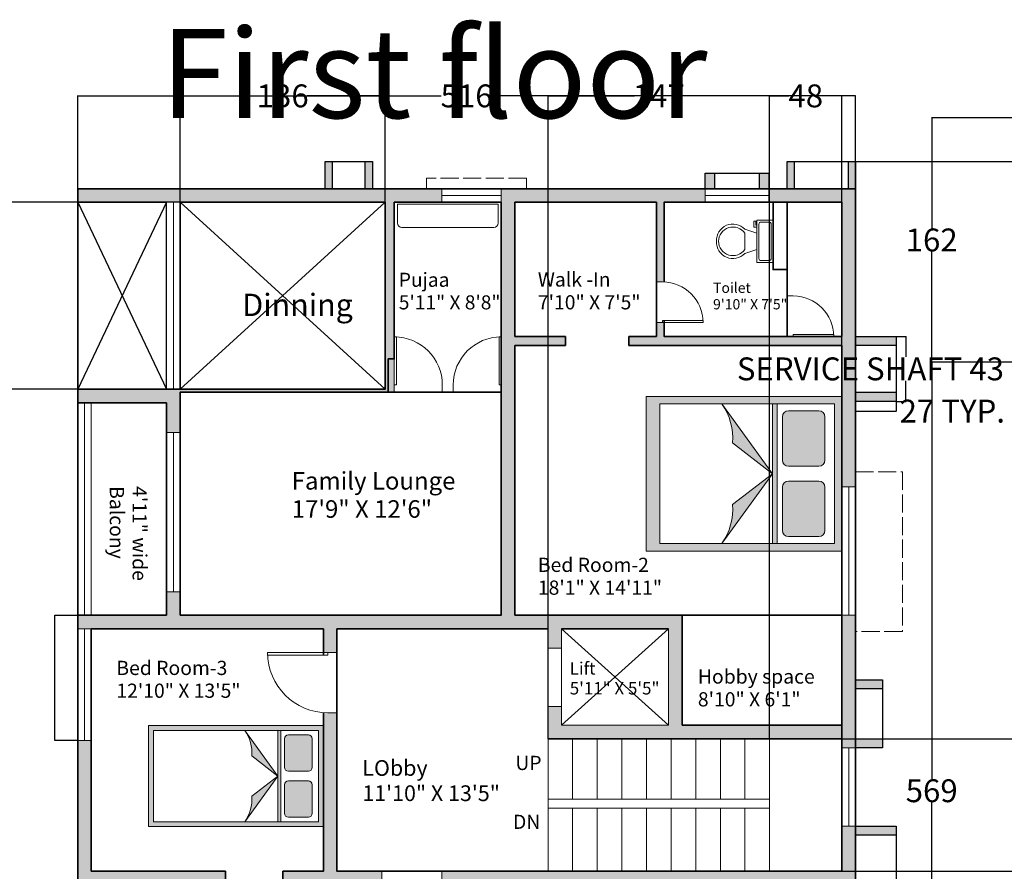
# Model space of a CAD drawing. Units: inches. Extents: x -828 to 1568, y -491 to 539.
# Tile 5 of 6: x 241 to 895, y -110 to 455. Entities that reach past the tile are written whole.
import ezdxf

# ---------------------------------------------------------------- set-up
doc = ezdxf.new("R2010")
doc.units = ezdxf.units.IN
doc.header["$MEASUREMENT"] = 0
doc.linetypes.add('ACAD_ISO02W100', pattern=[15, 12, -3])
for name, color, linetype, lineweight in [('A-ANNO-DIMS', 2, 'Continuous', 18), ('A-ANNO-TEXT', 7, 'Continuous', 18), ('A-ANNO-TITL', 7, 'Continuous', 35), ('A-AREA-IDEN', 7, 'Continuous', 18), ('A-DOOR', 3, 'Continuous', 18), ('A-FLOR-CASE', 9, 'Continuous', 18), ('A-FLOR-EDGE', 7, 'Continuous', 25), ('A-FLOR-EVTR', 4, 'Continuous', 18), ('A-FLOR-FIXT', 9, 'Continuous', 18), ('A-FLOR-OPEN', 8, 'Continuous', 13), ('A-FLOR-OVHD', 116, 'ACAD_ISO02W100', 13), ('A-FLOR-SHFT', 7, 'Continuous', 25), ('A-FLOR-STRS', 7, 'Continuous', 18), ('A-FURN', 8, 'Continuous', 18), ('A-FURN-PATT', 253, 'Continuous', 13), ('A-GLAZ', 4, 'Continuous', 18), ('A-WALL', 7, 'Continuous', 35), ('A-WALL-PATT', 8, 'Continuous', 13)]:
    doc.layers.add(name, color=color, linetype=linetype, lineweight=lineweight)
doc.styles.get("Standard").update_dxf_attribs({"font": 'arial.ttf'})
doc.dimstyles.get("Standard").update_dxf_attribs({"dimtxt": 15.18, "dimasz": 0.18, "dimexe": 0.18, "dimexo": 0.0625, "dimgap": 0.09, "dimtad": 0, "dimtih": 1, "dimtoh": 1, "dimdec": 0, "dimzin": 0, "dimdsep": 46, "dimlunit": 3, "dimtxsty": 'Standard', "dimcen": 0.09, "dimadec": 0, "dimazin": 0, "dimtfac": 1, "dimtdec": 0, "dimtofl": 0, "dimtmove": 0, "dimatfit": 3, "dimfxl": 1, "dimtolj": 1, "dimtzin": 0, "dimarcsym": 0})

# ---------------------------------------------------------------- blocks, each defined once
blk = doc.blocks.new('*U2')
for p, q in [((0, 0), (0, -6)), ((40, 0), (40, -6))]:
    blk.add_line(p, q)
blk.add_lwpolyline([(0, 0), (0, 40), (1.75, 40), (1.75, 0)], close=True)
blk.add_arc((0, 0), 40, 0, 90)
blk = doc.blocks.new('*U6')
for p, q in [((9.5, -6), (9.5, -2)), ((-10, -8.5), (-8, -8.5)), ((-10, -9.5), (-10, -8.5)), ((-7, -9.5), (-10, -9.5)), ((-8, -8.5), (-8, -8)), ((-7, -8), (-7, -9.5)), ((-4, -8), (-6, -14)), ((4, -8), (6, -14)), ((4, -14), (-4, -14))]:
    blk.add_line(p, q)
blk.add_lwpolyline([(10.5, -8), (10.5, 0), (-10.5, 0), (-10.5, -8)], close=True)
for points in [[(-9.5, -2), (-9.5, -6)], [(8.5, -1), (-8.5, -1)], [(-8.5, -7), (8.5, -7)]]:
    blk.add_lwpolyline(points)
for centre, radius, start, end in [((-8.625, -1.875), 0.8839, 81.8699, 188.1301), ((8.625, -1.875), 0.8839, 351.8699, 98.1301), ((-8.625, -6.125), 0.8839, 171.869898, 278.1301), ((8.625, -6.125), 0.8839, 261.8699, 8.1301), ((-0.4772, -19.9188), 8.0953, 133.01722, 273.38), ((0.0374, -19.8731), 7.127, 124.50543, 269.7), ((-0.0373, -19.8731), 7.127, 270.3, 55.4946), ((0.4773, -19.9188), 8.0953, 266.62, 46.9828)]:
    blk.add_arc(centre, radius, start, end)
blk = doc.blocks.new('SERVICE-SHAFT-43')
blk.add_line((26.86, 37.12), (26.86, 6))
for points in [[(0, 43.12), (26.86, 43.12), (26.86, 37.12), (0, 37.12)], [(0, 6), (26.86, 6), (26.86, 0), (0, 0)]]:
    blk.add_lwpolyline(points, close=True)
blk = doc.blocks.new('BED-FRAME-TURNBACK')
h = blk.add_hatch(color=256)
h.dxf.hatch_style = 1
h.paths.add_polyline_path([(0, 0), (115.93, 0), (115.93, 67.12), (0, 67.12)])
h.paths.add_polyline_path([(3.27, 63.85), (112.66, 63.85), (112.66, 3.27), (3.27, 3.27)], flags=16)
h = blk.add_hatch(color=256)
h.dxf.hatch_style = 1
h.paths.add_polyline_path([(63.77, 63.85, -0.182673), (68.41, 46.96), (85.81, 33.56)])
h.paths.add_polyline_path([(85.81, 33.56), (68.41, 20.16, -0.182673), (63.77, 3.27)])
h = blk.add_hatch(color=256)
h.dxf.hatch_style = 1
h.paths.add_polyline_path([(87.78, 33.56), (85.81, 33.56), (85.81, 3.27), (87.78, 3.27)])
h.paths.add_polyline_path([(87.78, 63.85), (85.81, 63.85), (85.81, 33.56), (87.78, 33.56)])
for p, q in [((85.81, 33.56), (63.77, 63.85)), ((85.81, 3.27), (85.81, 63.85)), ((87.78, 3.27), (87.78, 63.85)), ((85.81, 33.56), (68.41, 46.96))]:
    blk.add_line(p, q)
for points in [[(115.93, 0), (0, 0), (0, 67.12), (115.93, 67.12)], [(112.66, 3.27), (3.27, 3.27), (3.27, 63.85), (112.66, 63.85)]]:
    blk.add_lwpolyline(points, close=True)
blk.add_lwpolyline([(63.77, 3.27, 0.182673), (68.41, 20.16), (85.81, 33.56)], format="xyb", close=True)
blk.add_arc((43.75, 49.27), 24.77, 354.63295, 36.04187)
blk = doc.blocks.new('*D25')
at = {"layer": 'A-ANNO-DIMS', "color": 0, "lineweight": -2, "transparency": 16777216}
for p, q in [((822.84, 244.58), (829.43, 244.58)), ((829.25, 244.4), (829.25, 230.97)), ((829.25, 201.64), (829.25, 215.08)), ((822.84, 201.46), (829.43, 201.46))]:
    blk.add_line(p, q, dxfattribs=at)
at = {"layer": 'A-ANNO-DIMS', "color": 0, "lineweight": 20, "transparency": 16777216}
for points in [[(829.22, 244.4), (829.28, 244.4), (829.25, 244.58)], [(829.22, 201.64), (829.28, 201.64), (829.25, 201.46)]]:
    blk.add_solid(points, dxfattribs=at)
at = {"layer": 'DEFPOINTS', "color": 0, "lineweight": 20, "transparency": 16777216}
for p in [(822.78, 244.58), (829.25, 244.58), (822.78, 201.46)]:
    blk.add_point(p, dxfattribs=at)
at = {"layer": 'A-ANNO-DIMS', "color": 0, "transparency": 16777216, "insert": (829.25, 223.02), "char_height": 15.18, "attachment_point": 5}
blk.add_mtext('\\A1;SERVICE SHAFT 43 TYP.', dxfattribs=at)
blk = doc.blocks.new('*D26')
at = {"layer": 'A-ANNO-DIMS', "color": 0, "lineweight": -2, "transparency": 16777216}
for p, q in [((795.92, 201.4), (795.92, 194.82)), ((822.78, 201.4), (822.78, 194.82)), ((796.1, 195), (822.6, 195)), ((822.78, 195), (822.96, 195))]:
    blk.add_line(p, q, dxfattribs=at)
at = {"layer": 'A-ANNO-DIMS', "color": 0, "lineweight": 20, "transparency": 16777216}
for points in [[(796.1, 195.03), (796.1, 194.97), (795.92, 195)], [(822.6, 195.03), (822.6, 194.97), (822.78, 195)]]:
    blk.add_solid(points, dxfattribs=at)
at = {"layer": 'DEFPOINTS', "color": 0, "lineweight": 20, "transparency": 16777216}
for p in [(795.92, 201.46), (822.78, 201.46), (822.78, 195)]:
    blk.add_point(p, dxfattribs=at)
at = {"layer": 'A-ANNO-DIMS', "color": 0, "transparency": 16777216, "insert": (860.13, 195), "char_height": 15.18, "attachment_point": 5}
blk.add_mtext('\\A1;27 TYP.', dxfattribs=at)
blk = doc.blocks.new('*D40')
at = {"layer": 'A-ANNO-DIMS', "color": 0, "lineweight": -2, "transparency": 16777216}
for p, q in [((795.99, 360.63), (969.15, 360.63)), ((968.97, 360.45), (968.97, -20.38)), ((968.97, -416.57), (968.97, -35.74)), ((568.26, -416.75), (969.15, -416.75))]:
    blk.add_line(p, q, dxfattribs=at)
at = {"layer": 'A-ANNO-DIMS', "color": 0, "lineweight": 20, "transparency": 16777216}
for points in [[(968.94, 360.45), (969, 360.45), (968.97, 360.63)], [(968.94, -416.57), (969, -416.57), (968.97, -416.75)]]:
    blk.add_solid(points, dxfattribs=at)
at = {"layer": 'DEFPOINTS', "color": 0, "lineweight": 20, "transparency": 16777216}
for p in [(795.92, 360.63), (968.97, 360.63), (568.2, -416.75)]:
    blk.add_point(p, dxfattribs=at)
at = {"layer": 'A-ANNO-DIMS', "color": 0, "transparency": 16777216, "insert": (968.97, -28.06), "char_height": 15.18, "attachment_point": 5}
blk.add_mtext('\\A1;777.4', dxfattribs=at)
blk = doc.blocks.new('*D41')
at = {"layer": 'A-ANNO-DIMS', "color": 0, "lineweight": -2, "transparency": 16777216}
for p, q in [((279.92, 342.65), (279.92, 404.36)), ((280.1, 404.18), (521.07, 404.18)), ((795.74, 404.18), (554.78, 404.18)), ((795.92, 342.65), (795.92, 404.36))]:
    blk.add_line(p, q, dxfattribs=at)
at = {"layer": 'A-ANNO-DIMS', "color": 0, "lineweight": 20, "transparency": 16777216}
for points in [[(280.1, 404.21), (280.1, 404.15), (279.92, 404.18)], [(795.74, 404.21), (795.74, 404.15), (795.92, 404.18)]]:
    blk.add_solid(points, dxfattribs=at)
at = {"layer": 'DEFPOINTS', "color": 0, "lineweight": 20, "transparency": 16777216}
for p in [(795.92, 404.18), (279.92, 342.58), (795.92, 342.58)]:
    blk.add_point(p, dxfattribs=at)
at = {"layer": 'A-ANNO-DIMS', "color": 0, "transparency": 16777216, "insert": (537.92, 404.18), "char_height": 15.18, "attachment_point": 5}
blk.add_mtext('\\A1;516', dxfattribs=at)
blk = doc.blocks.new('*D42')
at = {"layer": 'A-ANNO-DIMS', "color": 0, "lineweight": -2, "transparency": 16777216}
for p, q in [((347.86, 209.58), (141.48, 209.58)), ((141.66, 209.4), (141.66, -76.07)), ((141.66, -377.24), (141.66, -91.76)), ((279.86, -377.42), (141.48, -377.42))]:
    blk.add_line(p, q, dxfattribs=at)
at = {"layer": 'A-ANNO-DIMS', "color": 0, "lineweight": 20, "transparency": 16777216}
for points in [[(141.63, 209.4), (141.69, 209.4), (141.66, 209.58)], [(141.63, -377.24), (141.69, -377.24), (141.66, -377.42)]]:
    blk.add_solid(points, dxfattribs=at)
at = {"layer": 'DEFPOINTS', "color": 0, "lineweight": 20, "transparency": 16777216}
for p in [(141.66, 209.58), (347.92, 209.58), (279.92, -377.42)]:
    blk.add_point(p, dxfattribs=at)
at = {"layer": 'A-ANNO-DIMS', "color": 0, "transparency": 16777216, "insert": (141.66, -83.92), "char_height": 15.18, "attachment_point": 5}
blk.add_mtext('\\A1;587', dxfattribs=at)
blk = doc.blocks.new('*D43')
at = {"layer": 'A-ANNO-DIMS', "color": 0, "lineweight": -2, "transparency": 16777216}
for p, q in [((347.92, 333.65), (347.92, 404.36)), ((348.1, 404.18), (399.78, 404.18)), ((483.74, 404.18), (432.06, 404.18)), ((483.92, 333.65), (483.92, 404.36))]:
    blk.add_line(p, q, dxfattribs=at)
at = {"layer": 'A-ANNO-DIMS', "color": 0, "lineweight": 20, "transparency": 16777216}
for points in [[(348.1, 404.21), (348.1, 404.15), (347.92, 404.18)], [(483.74, 404.21), (483.74, 404.15), (483.92, 404.18)]]:
    blk.add_solid(points, dxfattribs=at)
at = {"layer": 'DEFPOINTS', "color": 0, "lineweight": 20, "transparency": 16777216}
for p in [(483.92, 404.18), (347.92, 333.58), (483.92, 333.58)]:
    blk.add_point(p, dxfattribs=at)
at = {"layer": 'A-ANNO-DIMS', "color": 0, "transparency": 16777216, "insert": (415.92, 404.18), "char_height": 15.18, "attachment_point": 5}
blk.add_mtext('\\A1;136', dxfattribs=at)
blk = doc.blocks.new('*D44')
at = {"layer": 'A-ANNO-DIMS', "color": 0, "lineweight": -2, "transparency": 16777216}
for p, q in [((347.86, 333.58), (141.48, 333.58)), ((141.66, 333.4), (141.66, 279.3)), ((141.66, 209.76), (141.66, 263.87)), ((347.86, 209.58), (141.48, 209.58))]:
    blk.add_line(p, q, dxfattribs=at)
at = {"layer": 'A-ANNO-DIMS', "color": 0, "lineweight": 20, "transparency": 16777216}
for points in [[(141.63, 333.4), (141.69, 333.4), (141.66, 333.58)], [(141.63, 209.76), (141.69, 209.76), (141.66, 209.58)]]:
    blk.add_solid(points, dxfattribs=at)
at = {"layer": 'DEFPOINTS', "color": 0, "lineweight": 20, "transparency": 16777216}
for p in [(141.66, 333.58), (347.92, 333.58), (347.92, 209.58)]:
    blk.add_point(p, dxfattribs=at)
at = {"layer": 'A-ANNO-DIMS', "color": 0, "transparency": 16777216, "insert": (141.66, 271.58), "char_height": 15.18, "attachment_point": 5}
blk.add_mtext('\\A1;124', dxfattribs=at)
blk = doc.blocks.new('*D45')
at = {"layer": 'A-ANNO-DIMS', "color": 0, "lineweight": -2, "transparency": 16777216}
for p, q in [((591.92, -22.35), (591.92, 404.36)), ((592.1, 404.18), (649.28, 404.18)), ((738.74, 404.18), (681.57, 404.18)), ((738.92, -22.35), (738.92, 404.36))]:
    blk.add_line(p, q, dxfattribs=at)
at = {"layer": 'A-ANNO-DIMS', "color": 0, "lineweight": 20, "transparency": 16777216}
for points in [[(592.1, 404.21), (592.1, 404.15), (591.92, 404.18)], [(738.74, 404.21), (738.74, 404.15), (738.92, 404.18)]]:
    blk.add_solid(points, dxfattribs=at)
at = {"layer": 'DEFPOINTS', "color": 0, "lineweight": 20, "transparency": 16777216}
for p in [(738.92, 404.18), (591.92, -22.42), (738.92, -22.42)]:
    blk.add_point(p, dxfattribs=at)
at = {"layer": 'A-ANNO-DIMS', "color": 0, "transparency": 16777216, "insert": (665.42, 404.18), "char_height": 15.18, "attachment_point": 5}
blk.add_mtext('\\A1;147', dxfattribs=at)
blk = doc.blocks.new('*D46')
at = {"layer": 'A-ANNO-DIMS', "color": 0, "lineweight": -2, "transparency": 16777216}
for p, q in [((738.92, -22.35), (738.92, 404.36)), ((739.1, 404.18), (751.64, 404.18)), ((786.74, 404.18), (774.21, 404.18)), ((786.92, -22.35), (786.92, 404.36))]:
    blk.add_line(p, q, dxfattribs=at)
at = {"layer": 'A-ANNO-DIMS', "color": 0, "lineweight": 20, "transparency": 16777216}
for points in [[(739.1, 404.21), (739.1, 404.15), (738.92, 404.18)], [(786.74, 404.21), (786.74, 404.15), (786.92, 404.18)]]:
    blk.add_solid(points, dxfattribs=at)
at = {"layer": 'DEFPOINTS', "color": 0, "lineweight": 20, "transparency": 16777216}
for p in [(786.92, 404.18), (738.92, -22.42), (786.92, -22.42)]:
    blk.add_point(p, dxfattribs=at)
at = {"layer": 'A-ANNO-DIMS', "color": 0, "transparency": 16777216, "insert": (762.92, 404.18), "char_height": 15.18, "attachment_point": 5}
blk.add_mtext('\\A1;48', dxfattribs=at)
blk = doc.blocks.new('*D47')
at = {"layer": 'A-ANNO-DIMS', "color": 0, "lineweight": -2, "transparency": 16777216}
for p, q in [((786.99, -22.42), (969.15, -22.42)), ((968.97, -22.6), (968.97, -58.57)), ((968.97, -110.24), (968.97, -74.26)), ((786.99, -110.42), (969.15, -110.42))]:
    blk.add_line(p, q, dxfattribs=at)
at = {"layer": 'A-ANNO-DIMS', "color": 0, "lineweight": 20, "transparency": 16777216}
for points in [[(968.94, -22.6), (969, -22.6), (968.97, -22.42)], [(968.94, -110.24), (969, -110.24), (968.97, -110.42)]]:
    blk.add_solid(points, dxfattribs=at)
at = {"layer": 'DEFPOINTS', "color": 0, "lineweight": 20, "transparency": 16777216}
for p in [(786.92, -22.42), (968.97, -22.42), (786.92, -110.42)]:
    blk.add_point(p, dxfattribs=at)
at = {"layer": 'A-ANNO-DIMS', "color": 0, "transparency": 16777216, "insert": (968.97, -66.42), "char_height": 15.18, "attachment_point": 5}
blk.add_mtext('\\A1;88', dxfattribs=at)
blk = doc.blocks.new('*D53')
at = {"layer": 'A-ANNO-DIMS', "color": 0, "lineweight": -2, "transparency": 16777216}
for p, q in [((945.23, 389.57), (846.26, 389.57)), ((846.44, 389.39), (846.44, 316.41)), ((846.44, 227.74), (846.44, 300.73)), ((1093.6, 227.56), (846.26, 227.56))]:
    blk.add_line(p, q, dxfattribs=at)
at = {"layer": 'A-ANNO-DIMS', "color": 0, "lineweight": 20, "transparency": 16777216}
for points in [[(846.41, 389.39), (846.47, 389.39), (846.44, 389.57)], [(846.41, 227.74), (846.47, 227.74), (846.44, 227.56)]]:
    blk.add_solid(points, dxfattribs=at)
at = {"layer": 'DEFPOINTS', "color": 0, "lineweight": 20, "transparency": 16777216}
for p in [(945.29, 389.57), (846.44, 227.56), (1093.66, 227.56)]:
    blk.add_point(p, dxfattribs=at)
at = {"layer": 'A-ANNO-DIMS', "color": 0, "transparency": 16777216, "insert": (846.44, 308.57), "char_height": 15.18, "attachment_point": 5}
blk.add_mtext('\\A1;162', dxfattribs=at)
blk = doc.blocks.new('*D54')
at = {"layer": 'A-ANNO-DIMS', "color": 0, "lineweight": -2, "transparency": 16777216}
for p, q in [((1093.6, 227.56), (846.26, 227.56)), ((846.44, 227.38), (846.44, -49.1)), ((846.44, -341.26), (846.44, -64.78)), ((1093.6, -341.44), (846.26, -341.44))]:
    blk.add_line(p, q, dxfattribs=at)
at = {"layer": 'A-ANNO-DIMS', "color": 0, "lineweight": 20, "transparency": 16777216}
for points in [[(846.41, 227.38), (846.47, 227.38), (846.44, 227.56)], [(846.41, -341.26), (846.47, -341.26), (846.44, -341.44)]]:
    blk.add_solid(points, dxfattribs=at)
at = {"layer": 'DEFPOINTS', "color": 0, "lineweight": 20, "transparency": 16777216}
for p in [(846.44, 227.56), (1093.66, 227.56), (1093.66, -341.44)]:
    blk.add_point(p, dxfattribs=at)
at = {"layer": 'A-ANNO-DIMS', "color": 0, "transparency": 16777216, "insert": (846.44, -56.94), "char_height": 15.18, "attachment_point": 5}
blk.add_mtext('\\A1;569', dxfattribs=at)

msp = doc.modelspace()

# ---------------------------------------------------------------- hatches: boundary and pattern name
at = {"layer": 'A-FURN-PATT'}
h = msp.add_hatch(color=256, dxfattribs=at)
h.dxf.hatch_style = 1
h.paths.add_polyline_path([(657.0298, 204.7734), (657.0298, 102.1517), (786.9226, 102.1517), (786.9226, 204.7734)])
h.paths.add_polyline_path([(666.0298, 199.7734), (781.9226, 199.7734), (781.9226, 107.1517), (666.0298, 107.1517)], flags=16)
h = msp.add_hatch(color=256, dxfattribs=at)
h.dxf.hatch_style = 1
h.paths.add_polyline_path([(707.1718, 199.7734, -0.18267264), (714.2548, 173.9485), (740.8703, 153.4626)])
h.paths.add_polyline_path([(740.8703, 153.4626), (714.2548, 132.9767, -0.18267264), (707.1718, 107.1517)])
h = msp.add_hatch(color=256, dxfattribs=at)
h.dxf.hatch_style = 1
h.paths.add_polyline_path([(743.8703, 153.4626), (740.8703, 153.4626), (740.8703, 107.1517), (743.8703, 107.1517)])
h.paths.add_polyline_path([(743.8703, 199.7734), (740.8703, 199.7734), (740.8703, 153.4626), (743.8703, 153.4626)])
h = msp.add_hatch(color=256, dxfattribs=at)
h.dxf.hatch_style = 1
h.paths.add_polyline_path([(775.666, 191.2185, 0.41421356), (771.666, 195.2185), (751.4131, 195.2185, 0.41421356), (747.4131, 191.2185), (747.4131, 162.3574, 0.41421356), (751.4131, 158.3574), (771.666, 158.3574, 0.41421356), (775.666, 162.3574)])
h = msp.add_hatch(color=256, dxfattribs=at)
h.dxf.hatch_style = 1
h.paths.add_polyline_path([(747.4131, 115.7067, 0.41421356), (751.4131, 111.7067), (771.666, 111.7067, 0.41421356), (775.666, 115.7067), (775.666, 144.5678, 0.41421356), (771.666, 148.5678), (751.4131, 148.5678, 0.41421356), (747.4131, 144.5678)])
h = msp.add_hatch(color=256, dxfattribs=at)
h.dxf.hatch_style = 1
h.paths.add_polyline_path([(435.5603, -22.5037, 0.41421356), (432.9442, -19.8876), (419.6981, -19.8876, 0.41421356), (417.0819, -22.5037), (417.0819, -41.3799, 0.41421356), (419.6981, -43.9961), (432.9442, -43.9961, 0.41421356), (435.5603, -41.3799)])
h = msp.add_hatch(color=256, dxfattribs=at)
h.dxf.hatch_style = 1
h.paths.add_polyline_path([(417.0819, -71.8912, 0.41421356), (419.6981, -74.5074), (432.9442, -74.5074, 0.41421356), (435.5603, -71.8912), (435.5603, -53.015, 0.41421356), (432.9442, -50.3989), (419.6981, -50.3989, 0.41421356), (417.0819, -53.015)])
at = {"layer": 'A-WALL-PATT'}
h = msp.add_hatch(color=256, dxfattribs=at)
h.dxf.hatch_style = 1
h.paths.add_polyline_path([(795.9226, -243.7164), (786.9226, -243.7164), (786.9226, -278.4155), (699.9226, -278.4155), (699.9226, -262.0576), (693.9226, -262.0576), (693.9226, -284.4155), (786.9226, -284.4155), (786.9226, -368.4155), (634.9226, -368.4155), (634.9226, -184.8338), (628.9226, -184.8338), (628.9226, -368.4155), (541.609, -368.4155), (541.609, -377.4155), (795.9226, -377.4155)])
h.paths.add_polyline_path([(795.9226, -80.4153), (786.9226, -80.4153), (786.9226, -110.4155), (521.5942, -110.4155), (521.5942, -116.4155, -0.01876983), (521.4815, -119.4155), (693.9226, -119.4155), (693.9226, -222.9922), (699.9226, -222.9922), (699.9226, -119.4155), (786.9226, -119.4155), (786.9226, -208.3743), (795.9226, -208.3743)])
h.paths.add_polyline_path([(822.7802, -119.4155), (795.9226, -119.4155), (795.9226, -125.4155), (822.7802, -125.4155)])
h.paths.add_polyline_path([(822.7802, -80.4153), (795.9226, -80.4153), (795.9226, -86.4153), (822.7802, -86.4153)])
h.paths.add_polyline_path([(822.7802, -156.5366), (795.9226, -156.5366), (795.9226, -162.5366), (822.7802, -162.5366)])
h.paths.add_polyline_path([(813.7802, -208.3743), (795.9226, -208.3743), (795.9226, -214.3743), (813.7802, -214.3743)])
h.paths.add_polyline_path([(813.7802, -237.7164), (795.9226, -237.7164), (795.9226, -243.7164), (813.7802, -243.7164)])
h.paths.add_polyline_path([(568.196, -386.4155), (680.1012, -386.4155), (680.1012, -377.4155), (550.196, -377.4155), (550.196, -409.2892), (559.196, -409.2892), (559.196, -416.7473), (568.196, -416.7473)])
h.paths.add_polyline_path([(478.3036, -368.4155), (451.9226, -368.4155), (451.9226, -349.8576), (442.9226, -349.8576), (442.9226, -368.4155), (426.7914, -368.4155), (426.7914, -377.4155), (478.3036, -377.4155)])
h.paths.add_polyline_path([(550.196, -377.4155), (541.609, -377.4155), (426.7914, -377.4155), (426.7914, -377.6482), (312.8078, -377.4155), (307.3423, -386.4155), (550.196, -386.4155)])
h.paths.add_polyline_path([(312.8078, -377.4155), (312.8078, -368.4155), (288.9226, -368.4155), (288.9226, -351.7781), (279.9226, -351.7781), (279.9226, -377.4155), (279.9226, -416.7473), (288.9226, -416.7473)])
h.paths.add_polyline_path([(451.9226, -119.4155), (481.5942, -119.4155), (481.5942, -116.4155), (481.5942, -110.4155), (451.9226, -110.4155), (451.9226, -5.2313), (445.9226, -5.2313, -0.01876983), (442.9226, -5.1187), (442.9226, -110.4155), (416.0227, -110.4155), (416.0227, -119.4155), (442.9226, -119.4155), (442.9226, -241.4155), (377.9226, -241.4155), (377.9226, -196.3369), (371.9226, -196.3369), (371.9226, -241.4155), (288.9226, -241.4155), (279.9226, -241.4155), (279.9226, -273.9916), (288.9226, -273.9916), (288.9226, -250.4155), (442.9226, -250.4155), (442.9226, -286.5741), (451.9226, -286.5741)])
h.paths.add_polyline_path([(377.9226, -110.4155), (288.9226, -110.4155), (288.9226, -23.5133), (279.9226, -23.5133), (279.9226, -209.5643), (288.9226, -209.5643), (288.9226, -119.4155), (371.9226, -119.4155), (371.9226, -163.1368), (377.9226, -163.1368)], flags=17)
h.paths.add_polyline_path([(279.9226, -200.5643), (259.4345, -200.5643), (259.4345, -209.5643), (279.9226, -209.5643)])
h.paths.add_polyline_path([(279.9226, -163.4155), (259.4345, -163.4155), (259.4345, -172.4155), (279.9226, -172.4155)])
h.paths.add_polyline_path([(680.9226, 59.5845), (569.9226, 59.5845), (569.9226, 238.5845), (603.4634, 238.5845), (603.4634, 244.5845), (569.9226, 244.5845), (569.9226, 333.5845), (663.9226, 333.5845), (663.9226, 280.6911), (667.9428, 280.6911, -0.00914136), (668.9226, 280.6732), (668.9226, 333.5845), (696.1553, 333.5845), (696.1553, 342.5845), (560.9226, 342.5845), (560.9226, 333.5845), (560.9226, 229.5845), (560.9226, 212.3675), (560.9226, 207.5845), (560.9226, 59.5845), (347.9226, 59.5845), (347.9226, 75.0877), (338.9226, 75.0877), (338.9226, 59.5845), (279.9226, 59.5845), (279.9226, 50.5845), (288.9226, 50.5845), (442.9226, 50.5845), (442.9226, 34.7687), (445.9226, 34.7687), (451.9226, 34.7687), (451.9226, 50.5845), (591.9226, 50.5845), (591.9226, 37.5639), (600.9226, 37.5639), (600.9226, 50.5845), (671.9226, 50.5845), (671.9226, -13.4155), (600.9226, -13.4155), (600.9226, -1.0868), (591.9226, -1.0868), (591.9226, -22.4155), (680.9226, -22.4155), (786.9226, -22.4155), (786.9226, -13.4155), (680.9226, -13.4155)])
h.paths.add_polyline_path([(813.7802, -22.4155), (795.9226, -22.4155), (795.9226, -28.4155), (813.7802, -28.4155)])
h.paths.add_polyline_path([(795.9226, 59.5845), (786.9226, 59.5845), (786.9226, -13.4155), (786.9226, -22.4155), (786.9226, -28.4155), (795.9226, -28.4155), (795.9226, -22.4155)])
h.paths.add_polyline_path([(813.7802, 16.5847), (795.9226, 16.5847), (795.9226, 10.5847), (813.7802, 10.5847)])
h.paths.add_polyline_path([(795.9226, 342.5845), (791.2302, 342.5845), (738.4317, 342.5845), (738.4317, 333.5845), (786.9226, 333.5845), (786.9226, 244.5845), (668.9226, 244.5845), (668.9226, 253.8895), (667.9428, 253.8895), (663.9226, 253.8895), (663.9226, 244.5845), (645.6004, 244.5845), (645.6004, 238.5845), (786.9226, 238.5845), (786.9226, 144.7189), (795.9226, 144.7189)])
h.paths.add_polyline_path([(822.7802, 207.4634), (795.9226, 207.4634), (795.9226, 201.4634), (822.7802, 201.4634)])
h.paths.add_polyline_path([(822.7802, 244.5845), (795.9226, 244.5845), (795.9226, 238.5845), (822.7802, 238.5845)])
h.paths.add_polyline_path([(347.9226, 207.5845), (386.8215, 207.5845), (485.9226, 207.5845), (485.9226, 229.5845), (489.9226, 229.5845), (489.9226, 244.2539), (489.9226, 333.5845), (521.5185, 333.5845), (521.5185, 342.5845), (279.9226, 342.5845), (279.9226, 333.5845), (338.9226, 333.5845), (347.9226, 333.5845), (483.9226, 333.5845), (483.9226, 209.5845), (386.8215, 209.5845), (338.9226, 209.5845), (279.9226, 209.5845), (279.9226, 200.5845), (288.9226, 200.5845), (338.9226, 200.5845), (338.9226, 180.8391), (347.9226, 180.8391)])
h.paths.add_polyline_path([(795.9226, 360.6319), (791.2302, 360.6319), (791.2302, 342.5845), (795.9226, 342.5845)])
h.paths.add_polyline_path([(755.2954, 360.6319), (750.6031, 360.6319), (750.6031, 342.5845), (755.2954, 342.5845)])
h.paths.add_polyline_path([(738.4317, 352.9518), (732.1778, 352.9518), (732.1778, 342.5845), (738.4317, 342.5845)])
h.paths.add_polyline_path([(702.4092, 352.9518), (696.1553, 352.9518), (696.1553, 342.5845), (702.4092, 342.5845)])
h.paths.add_polyline_path([(475.4018, 360.6319), (470.7095, 360.6319), (470.7095, 342.5845), (475.4018, 342.5845)])
h.paths.add_polyline_path([(448.7297, 360.6319), (444.0374, 360.6319), (444.0374, 342.5845), (448.7297, 342.5845)])
h.paths.add_polyline_path([(489.9226, 229.5845), (485.9226, 229.5845), (485.9226, 207.5845), (489.9226, 207.5845), (489.9226, 212.3675)], flags=17)
h.paths.add_polyline_path([(708.7018, -15.9815), (795.2211, -15.9815), (795.2211, -1.5493), (708.7018, -1.5493)], flags=9)
h.paths.add_polyline_path([(598.5172, 15.6725), (685.0365, 15.6725), (685.0365, 30.1047), (598.5172, 30.1047)], flags=25)
h.paths.add_polyline_path([(598.5188, 30.8165), (677.2194, 30.8165), (677.2194, 45.2391), (598.5188, 45.2391)], flags=25)

# ---------------------------------------------------------------- linework, layer by layer
at = {"layer": 'A-FLOR-CASE'}
msp.add_lwpolyline([(492.0191, 332.3212), (558.893, 332.3212), (558.893, 319.8375, -0.41421356), (555.893, 316.8375), (495.0191, 316.8375, -0.41421356), (492.0191, 319.8375)], format="xyb", close=True, dxfattribs=at)
at = {"layer": 'A-FLOR-EDGE'}
msp.add_lwpolyline([(279.9226, -23.5133), (264.8323, -23.5133), (264.8323, 59.5845), (279.9226, 59.5845), (279.9226, 333.5845), (338.9226, 333.5845), (279.9226, 333.5845), (338.9226, 209.5845), (338.9226, 333.5845), (279.9226, 209.5845)], dxfattribs=at)
at = {"layer": 'A-FLOR-EVTR'}
for points in [[(671.9226, 50.5845), (671.9226, -13.4155), (600.9226, -13.4155), (671.9226, 50.5845), (671.9226, -13.4155), (600.9226, 50.5845), (600.9226, -13.4155), (600.9226, 50.5845)], [(600.9226, -1.0868), (591.9226, -1.0868), (591.9226, 37.5639), (600.9226, 37.5639)]]:
    msp.add_lwpolyline(points, close=True, dxfattribs=at)
at = {"layer": 'A-FLOR-OPEN'}
for p, q in [((347.9226, 209.5845), (483.9226, 333.5845)), ((483.9226, 209.5845), (347.9226, 333.5845)), ((483.9226, 333.5845), (483.9226, 209.5845))]:
    msp.add_line(p, q, dxfattribs=at)
at = {"layer": 'A-FLOR-OVHD'}
for points in [[(577.6682, 342.5845), (577.6682, 349.5448), (511.2721, 349.5448), (511.2721, 342.5845)], [(795.9226, 154.6955), (826.986, 154.6955), (826.986, 48.6302), (795.9226, 48.6302)]]:
    msp.add_lwpolyline(points, dxfattribs=at)
at = {"layer": 'A-FLOR-SHFT'}
for p, q in [((448.7297, 360.6319), (470.7095, 360.6319)), ((755.2954, 360.6319), (791.2302, 360.6319)), ((702.4092, 352.9518), (732.1778, 352.9518)), ((813.7802, 10.5847), (813.7802, -22.4155)), ((822.7802, -86.4153), (822.7802, -119.4155))]:
    msp.add_line(p, q, dxfattribs=at)
for points in [[(448.7297, 342.5845), (444.0374, 342.5845), (444.0374, 360.6319), (448.7297, 360.6319)], [(475.4018, 342.5845), (470.7095, 342.5845), (470.7095, 360.6319), (475.4018, 360.6319)], [(755.2954, 342.5845), (750.6031, 342.5845), (750.6031, 360.6319), (755.2954, 360.6319)], [(795.9226, 342.5845), (791.2302, 342.5845), (791.2302, 360.6319), (795.9226, 360.6319)], [(702.4092, 342.5845), (696.1553, 342.5845), (696.1553, 352.9518), (702.4092, 352.9518)], [(738.4317, 342.5845), (732.1778, 342.5845), (732.1778, 352.9518), (738.4317, 352.9518)], [(795.9226, -80.4153), (822.7802, -80.4153), (822.7802, -86.4153), (795.9226, -86.4153)]]:
    msp.add_lwpolyline(points, close=True, dxfattribs=at)
for points in [[(786.9226, 10.5847), (786.9226, 16.5847)], [(795.9226, 16.5847), (813.7802, 16.5847), (813.7802, 10.5847), (795.9226, 10.5847)], [(795.9226, -22.4155), (813.7802, -22.4155), (813.7802, -28.4155), (795.9226, -28.4155)]]:
    msp.add_lwpolyline(points, dxfattribs=at)
at = {"layer": 'A-FLOR-STRS'}
for p, q in [((608.2561, -62.4655), (608.2561, -22.4155)), ((624.5896, -62.4655), (624.5896, -22.4155)), ((640.9231, -62.4655), (640.9231, -22.4155)), ((657.2566, -62.4655), (657.2566, -22.4155)), ((673.5901, -62.4655), (673.5901, -22.4155)), ((689.9236, -62.4655), (689.9236, -22.4155)), ((706.2571, -62.4655), (706.2571, -22.4155)), ((722.5906, -62.4655), (722.5906, -22.4155)), ((738.9241, -62.4655), (591.9226, -62.4655))]:
    msp.add_line(p, q, dxfattribs=at)
msp.add_lwpolyline([(591.9226, -22.4155), (591.9226, 50.5845), (591.9226, -13.4155), (591.9226, -22.4155), (591.9226, -68.4655), (591.9226, -110.4155), (591.9226, -68.4655), (738.9241, -68.4655), (738.9241, -110.4155), (738.9241, -22.4155)], dxfattribs=at)
for points in [[(608.2561, -110.4155), (608.2561, -68.4655)], [(624.5896, -110.4155), (624.5896, -68.4655)], [(640.9231, -110.4155), (640.9231, -68.4655)], [(657.2566, -110.4155), (657.2566, -68.4655)], [(673.5901, -110.4155), (673.5901, -68.4655)], [(689.9236, -110.4155), (689.9236, -68.4655)], [(706.2571, -110.4155), (706.2571, -68.4655)], [(722.5906, -110.4155), (722.5906, -68.4655)]]:
    msp.add_lwpolyline(points, close=True, dxfattribs=at)
at = {"layer": 'A-FURN'}
for p, q in [((740.8703, 153.4626), (707.1718, 199.7734)), ((740.8703, 107.1517), (740.8703, 199.7734)), ((743.8703, 107.1517), (743.8703, 199.7734)), ((740.8703, 153.4626), (714.2548, 173.9485))]:
    msp.add_line(p, q, dxfattribs=at)
for points in [[(786.9226, 102.1517), (657.0298, 102.1517), (657.0298, 204.7734), (786.9226, 204.7734)], [(781.9226, 107.1517), (666.0298, 107.1517), (666.0298, 199.7734), (781.9226, 199.7734)]]:
    msp.add_lwpolyline(points, close=True, dxfattribs=at)
for points in [[(771.666, 158.3574), (751.4131, 158.3574, -0.41421356), (747.4131, 162.3574), (747.4131, 191.2185, -0.41421356), (751.4131, 195.2185), (771.666, 195.2185, -0.41421356), (775.666, 191.2185), (775.666, 162.3574, -0.41421356)], [(707.1718, 107.1517, 0.18267264), (714.2548, 132.9767), (740.8703, 153.4626)], [(771.666, 148.5678), (751.4131, 148.5678, 0.41421356), (747.4131, 144.5678), (747.4131, 115.7067, 0.41421356), (751.4131, 111.7067), (771.666, 111.7067, 0.41421356), (775.666, 115.7067), (775.666, 144.5678, 0.41421356)], [(432.9442, -43.9961), (419.6981, -43.9961, -0.41421356), (417.0819, -41.3799), (417.0819, -22.5037, -0.41421356), (419.6981, -19.8876), (432.9442, -19.8876, -0.41421356), (435.5603, -22.5037), (435.5603, -41.3799, -0.41421356)], [(432.9442, -50.3989), (419.6981, -50.3989, 0.41421356), (417.0819, -53.015), (417.0819, -71.8912, 0.41421356), (419.6981, -74.5074), (432.9442, -74.5074, 0.41421356), (435.5603, -71.8912), (435.5603, -53.015, 0.41421356)]]:
    msp.add_lwpolyline(points, format="xyb", close=True, dxfattribs=at)
msp.add_arc((676.5494, 177.4908), 37.8714, 354.6329524, 36.0418698, dxfattribs=at)
at = {"layer": 'A-GLAZ'}
for p, q in [((343.4226, 333.5845), (343.4226, 209.5845)), ((696.1553, 338.0845), (738.4317, 338.0845)), ((284.4226, 59.5845), (284.4226, 200.5845)), ((343.4226, 75.0877), (343.4226, 180.8391)), ((791.4226, 59.5845), (791.4226, 144.7189)), ((284.4226, -23.5133), (284.4226, 50.5845)), ((791.4226, -80.4153), (791.4226, -28.4155))]:
    msp.add_line(p, q, dxfattribs=at)
msp.add_lwpolyline([(560.9226, 244.5845), (560.9226, 333.5845), (560.9226, 342.5845), (521.5185, 342.5845), (521.5185, 333.5845), (560.9226, 333.5845), (560.9226, 338.0845), (521.5185, 338.0845)], dxfattribs=at)
for points in [[(738.4317, 342.5845), (696.1553, 342.5845), (696.1553, 333.5845), (738.4317, 333.5845)], [(347.9226, 209.5845), (338.9226, 209.5845), (338.9226, 333.5845), (347.9226, 333.5845)], [(279.9226, 200.5845), (288.9226, 200.5845), (288.9226, 59.5845), (279.9226, 59.5845)], [(338.9226, 180.8391), (347.9226, 180.8391), (347.9226, 75.0877), (338.9226, 75.0877)], [(786.9226, 59.5845), (795.9226, 59.5845), (795.9226, 144.7189), (786.9226, 144.7189)], [(288.9226, 50.5845), (279.9226, 50.5845), (279.9226, -23.5133), (288.9226, -23.5133)], [(795.9226, -28.4155), (786.9226, -28.4155), (786.9226, -80.4153), (795.9226, -80.4153)]]:
    msp.add_lwpolyline(points, close=True, dxfattribs=at)
at = {"layer": 'A-WALL'}
for p, q in [((279.9226, 342.5845), (795.9226, 342.5845)), ((795.9226, 342.5845), (795.9226, -377.4155)), ((347.9226, 333.5845), (347.9226, 209.5845)), ((347.9226, 333.5845), (483.9226, 333.5845)), ((483.9226, 333.5845), (483.9226, 229.5845)), ((569.9226, 333.5845), (663.9226, 333.5845)), ((663.9226, 333.5845), (663.9226, 244.5845)), ((750.6031, 288.9005), (750.6031, 244.5845)), ((569.9226, 244.5845), (603.4634, 244.5845)), ((603.4634, 244.5845), (603.4634, 238.5845)), ((645.6004, 238.5845), (645.6004, 244.5845)), ((645.6004, 244.5845), (663.9226, 244.5845)), ((569.9226, 238.5845), (603.4634, 238.5845)), ((569.9226, 238.5845), (569.9226, 59.5845)), ((645.6004, 238.5845), (786.9226, 238.5845)), ((786.9226, 238.5845), (786.9226, 59.5845)), ((338.9226, 209.5845), (279.9226, 209.5845)), ((279.9226, 209.5845), (279.9226, 200.5845)), ((347.9226, 209.5845), (347.9226, 209.5845)), ((485.9226, 207.5845), (560.9226, 207.5845)), ((279.9226, 200.5845), (279.9226, 200.5845)), ((279.9226, 200.5845), (338.9226, 200.5845)), ((338.9226, 200.5845), (338.9226, 59.5845)), ((279.9226, 59.5845), (338.9226, 59.5845)), ((338.9226, 59.5845), (279.9226, 59.5845)), ((279.9226, 59.5845), (279.9226, 59.5845)), ((569.9226, 59.5845), (786.9226, 59.5845)), ((786.9226, 59.5845), (680.9226, 59.5845)), ((680.9226, 59.5845), (680.9226, -13.4155)), ((786.9226, -13.4155), (786.9226, 59.5845)), ((288.9226, 50.5845), (442.9226, 50.5845)), ((288.9226, 50.5845), (288.9226, -110.4155)), ((442.9226, 50.5845), (442.9226, 33.0187)), ((451.9226, 50.5845), (591.9226, 50.5845)), ((451.9226, 50.5845), (591.9226, 50.5845)), ((600.9226, 50.5845), (671.9226, 50.5845)), ((680.9226, -13.4155), (786.9226, -13.4155)), ((288.9226, -110.4155), (377.9226, -110.4155)), ((377.9226, -163.1368), (377.9226, -110.4155))]:
    msp.add_line(p, q, dxfattribs=at)
for points in [[(279.9226, 333.5845), (279.9226, 342.5845), (279.9226, 50.5845), (279.9226, -377.4155), (279.9226, -416.7473), (288.9226, -416.7473)], [(560.9226, 333.5845), (489.9226, 333.5845), (489.9226, 229.5845), (485.9226, 229.5845), (485.9226, 207.5845), (386.8215, 207.5845), (347.9226, 207.5845), (347.9226, 59.5845), (347.9226, 207.5845)], [(560.9226, 229.5845), (560.9226, 229.5845), (560.9226, 333.5845), (560.9226, 59.5845), (347.9226, 59.5845)], [(668.9226, 255.0621), (668.9226, 244.5845), (786.9226, 244.5845), (786.9226, 333.5845), (786.9226, 244.5845)], [(786.9226, 333.5845), (668.9226, 333.5845), (668.9226, 280.6732)], [(483.9226, 229.5845), (483.9226, 209.5845), (386.8215, 209.5845), (338.9226, 209.5845)], [(451.9226, 50.5845), (451.9226, -110.4155), (786.9226, -110.4155), (786.9226, 50.5845)], [(442.9226, -241.4155), (442.9226, -119.4155), (416.0227, -119.4155), (416.0227, -110.4155), (442.9226, -110.4155), (442.9226, -5.1187)], [(786.9226, -28.4155), (786.9226, -22.4155), (680.9226, -22.4155), (591.9226, -22.4155), (680.9226, -22.4155)]]:
    msp.add_lwpolyline(points, dxfattribs=at)
for points in [[(569.9226, 333.5845), (569.9226, 244.5845)], [(750.6031, 333.5845), (741.2386, 333.5845), (741.2386, 288.9005), (750.6031, 288.9005)]]:
    msp.add_lwpolyline(points, close=True, dxfattribs=at)

# ---------------------------------------------------------------- block references
at = {"layer": 'A-DOOR', "xscale": -0.670039174459592, "yscale": 0.670039174459592, "zscale": 0.670039174459592, "rotation": 270}
for p in [(667.9428, 253.8895), (754.6233, 244.5845)]:
    msp.add_blockref('*U2', p, dxfattribs=at)
at = {"layer": 'A-DOOR', "yscale": 0.7971596692493578, "zscale": 0.7971596692493578}
for p, xscale in [((489.9226, 212.3675), 0.7971596692493578), ((560.9226, 212.3675), -0.7971596692493578)]:
    msp.add_blockref('*U2', p, dxfattribs=dict(at, xscale=xscale))
at = {"layer": 'A-DOOR', "xscale": -1}
for p, rotation in [((445.9226, 34.7687), 90), ((481.5942, -116.4155), 180)]:
    msp.add_blockref('*U2', p, dxfattribs=dict(at, rotation=rotation))
at = {"layer": 'A-FLOR-FIXT', "xscale": 1.340317743543512, "yscale": 1.340317743543512, "zscale": 1.340317743543512, "rotation": 270}
msp.add_blockref('*U6', (741.2386, 307.6692), dxfattribs=at)
at = {"layer": 'A-FLOR-SHFT'}
msp.add_blockref('SERVICE-SHAFT-43', (795.923, 201.463), dxfattribs=at)
at = {"layer": 'A-FURN'}
msp.add_blockref('BED-FRAME-TURNBACK', (326.989, -80.757), dxfattribs=at)

# ---------------------------------------------------------------- texts
at = {"layer": 'A-ANNO-TEXT'}
for s, p in [('UP', (570.2587, -43.1911)), ('DN', (568.7066, -82.2876))]:
    msp.add_text(s, height=9.42222, dxfattribs=at).set_placement(p)
at = {"layer": 'A-ANNO-TITL'}
msp.add_text('First floor', height=59.169316, dxfattribs=at).set_placement((334.9613, 389.4521))
at = {"layer": 'A-AREA-IDEN'}
for s, height, p in [('Walk -In', 9.42222, (585.1885, 277.6327)), ('Pujaa', 9.33198, (492.9426, 277.4877)), ('Toilet', 6.81219, (701.4054, 273.4399)), ('Dinning', 14.8042, (389.1199, 258.09)), ('5\'11" X 8\'8"', 9.331978, (492.9426, 262.4967)), ('7\'10" X 7\'5"', 9.422225, (585.1885, 262.4967)), ('9\'10" X 7\'5"', 6.812193, (701.4054, 262.4967)), ('Family Lounge', 11.654508, (421.9245, 142.9192)), ('17\'9" X 12\'6"', 11.654508, (421.9245, 124.1973)), ('Bed Room-2', 9.42222, (585.1885, 88.2623)), ('18\'1" X 14\'11"', 9.422225, (585.1885, 73.1263)), ('Bed Room-3', 9.42222, (305.5746, 19.8598)), ('Lift ', 8.23009, (606.3657, 20.1487)), ('Hobby space', 9.422225, (691.3382, 14.1539)), ('12\'10" X 13\'5"', 9.422225, (305.5746, 4.7238)), ('5\'11" X 5\'5"', 8.230085, (606.3657, 6.9278)), ('8\'10" X 6\'1"', 9.422225, (691.3382, -0.982)), ('LObby', 10.43699, (468.7505, -47.0443)), ('11\'10" X 13\'5"', 10.436991, (468.7505, -63.8104))]:
    msp.add_text(s, height=height, dxfattribs=at).set_placement(p)
for s, p in [('Balcony', (301.2262, 145.2205)), ('4\'11" wide', (316.3622, 145.2205))]:
    msp.add_text(s, height=9.42222, rotation=270, dxfattribs=at).set_placement(p)

# ---------------------------------------------------------------- dimensions: what is measured, and where the dimension line sits
at = {"layer": 'A-ANNO-DIMS'}
for base, p1, p2, picture, middle in [((795.9226, 404.1819), (279.9226, 342.5845), (795.9226, 342.5845), '*D41', (537.9226, 404.1819)), ((483.9226, 404.1819), (347.9226, 333.5845), (483.9226, 333.5845), '*D43', (415.9226, 404.1819)), ((738.9241, 404.1819), (591.9226, -22.4155), (738.9241, -22.4155), '*D45', (665.4233, 404.1819)), ((786.9226, 404.1819), (738.9241, -22.4155), (786.9226, -22.4155), '*D46', (762.9233, 404.1819))]:
    dim = msp.add_linear_dim(base=base, p1=p1, p2=p2, dimstyle='Standard', override={"dimdec": 0, "dimlfac": 1, "dimrnd": 0, "dimzin": 0, "dimdsep": 46, "dimlunit": 2}, dxfattribs=at)
    dim.commit()
    dim.dimension.update_dxf_attribs({"geometry": picture, "text_midpoint": middle})
for base, p1, p2, override, picture, middle in [((846.4381, 227.5603), (945.2883, 389.5728), (1093.6584, 227.5603), {"dimdec": 0, "dimlfac": 1, "dimrnd": 0, "dimzin": 0, "dimdsep": 46, "dimlunit": 2}, '*D53', (846.4381, 308.5666)), ((968.971, 360.6319), (568.196, -416.7473), (795.9226, 360.6319), {"dimdec": 1, "dimlfac": 1, "dimrnd": 0, "dimzin": 0, "dimdsep": 46, "dimlunit": 2}, '*D40', (968.971, -28.0577)), ((141.6607, 333.5845), (347.9226, 209.5845), (347.9226, 333.5845), {"dimdec": 0, "dimlfac": 1, "dimrnd": 0, "dimzin": 0, "dimdsep": 46, "dimlunit": 2}, '*D44', (141.6607, 271.5845)), ((846.4381, 227.5603), (1093.6584, -341.4397), (1093.6584, 227.5603), {"dimdec": 0, "dimlfac": 1, "dimrnd": 0, "dimzin": 0, "dimdsep": 46, "dimlunit": 2}, '*D54', (846.4381, -56.9397)), ((141.6607, 209.5845), (279.9226, -377.4155), (347.9226, 209.5845), {"dimdec": 0, "dimlfac": 1, "dimrnd": 0, "dimzin": 0, "dimdsep": 46, "dimlunit": 2}, '*D42', (141.6607, -83.9155)), ((968.971, -22.4155), (786.9226, -110.4155), (786.9226, -22.4155), {"dimdec": 0, "dimlfac": 1, "dimrnd": 0, "dimzin": 0, "dimdsep": 46, "dimlunit": 2}, '*D47', (968.971, -66.4155))]:
    dim = msp.add_linear_dim(base=base, p1=p1, p2=p2, angle=90, dimstyle='Standard', override=override, dxfattribs=at)
    dim.commit()
    dim.dimension.update_dxf_attribs({"geometry": picture, "text_midpoint": middle})
dim = msp.add_linear_dim(base=(829.2484, 244.5845), p1=(822.7802, 201.4634), p2=(822.7802, 244.5845), angle=90, text='SERVICE SHAFT <> TYP.', dimstyle='Standard', override={"dimdec": 0, "dimlfac": 1, "dimrnd": 0, "dimzin": 0, "dimdsep": 46, "dimlunit": 2}, dxfattribs=at)
dim.commit()
dim.dimension.update_dxf_attribs({"geometry": '*D25', "text_midpoint": (829.2484, 223.0239)})
dim = msp.add_linear_dim(base=(822.7802, 194.9952), p1=(795.9226, 201.4634), p2=(822.7802, 201.4634), text='<> TYP.', dimstyle='Standard', override={"dimdec": 0, "dimlfac": 1, "dimrnd": 0, "dimzin": 0, "dimdsep": 46, "dimlunit": 2}, dxfattribs=at)
dim.commit()
dim.dimension.update_dxf_attribs({"geometry": '*D26', "text_midpoint": (860.1252, 194.9952)})

doc.saveas('drawing.dxf')
